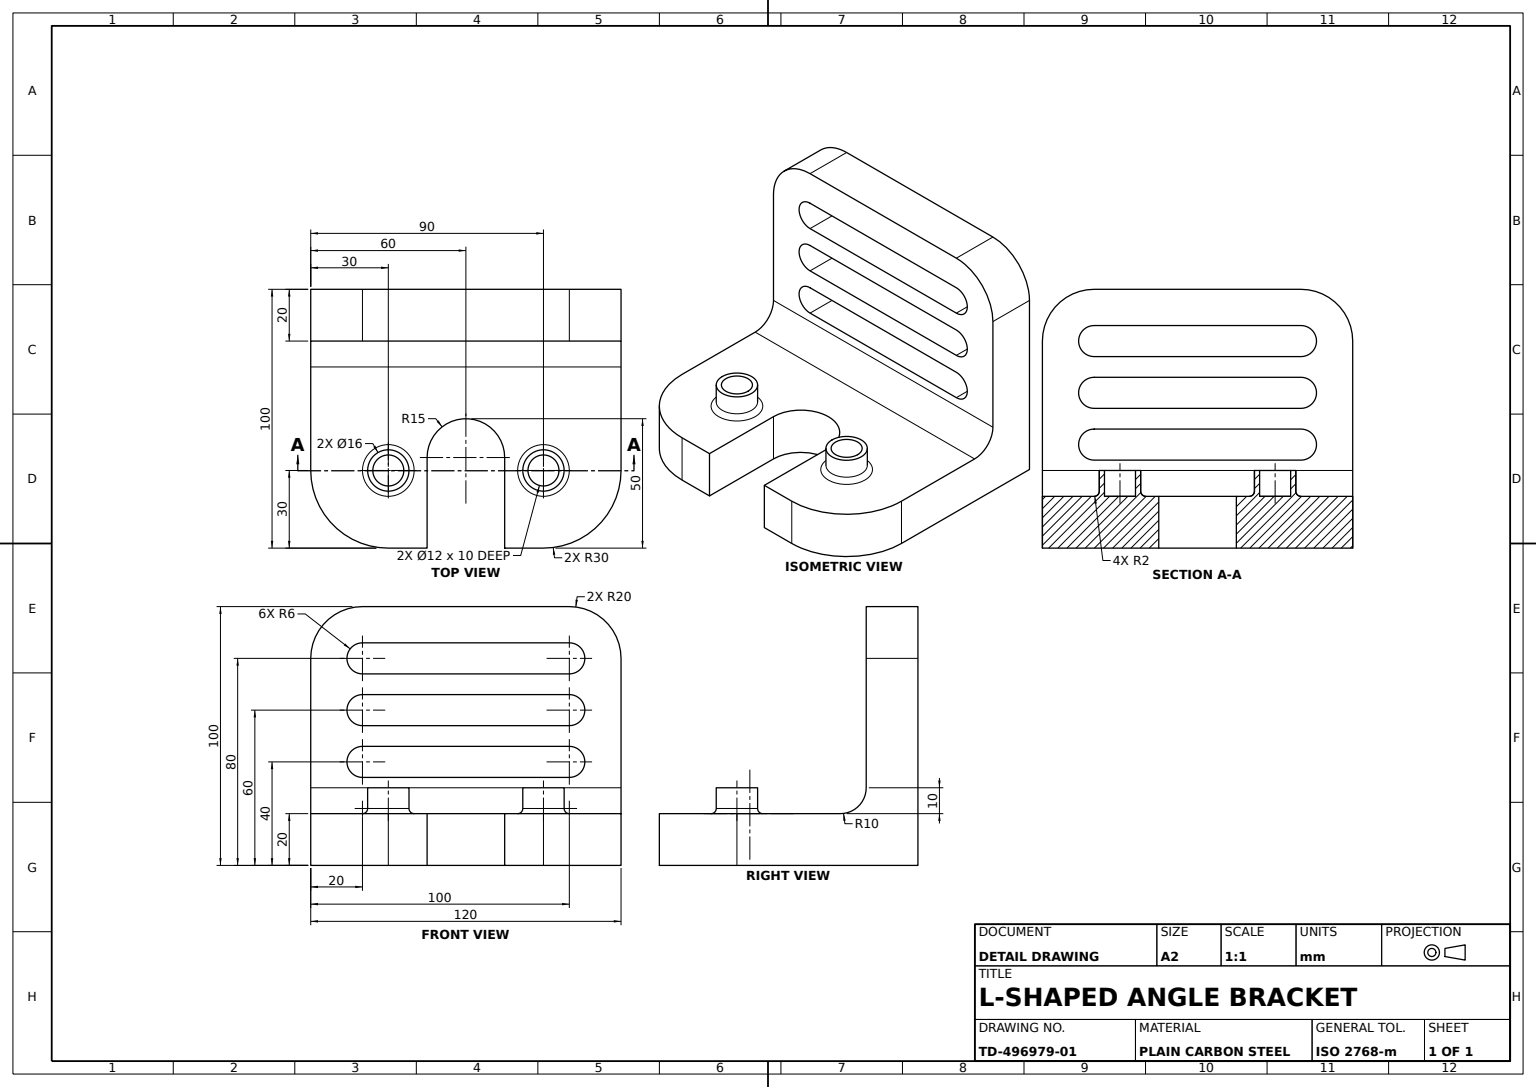
SolidWorks part; units mm, degrees
material "Plain Carbon Steel"
ref_plane "Front Plane" through (0, 0, 0) normal (0, 0, 1) x (1, 0, 0)
ref_plane "Top Plane" through (0, 0, 0) normal (0, 1, 0) x (1, 0, 0)
ref_plane "Right Plane" through (0, 0, 0) normal (1, 0, 0) x (0, 0, -1)
sketch "Bracket L Profile" plane through (0, 0, 0) normal (0, 0, 1) x (1, 0, 0)
  line L1 (0, 0) -> (20, 0)
  line L2 (0, 0) -> (0, -100)
  line L3 (0, -100) -> (20, -100)
  line L4 (20, 0) -> (20, -70)
  line L5 (0, -100) -> (100, -100)
  line L6 (0, -100) -> (0, -80)
  line L7 (30, -80) -> (100, -80)
  line L8 (100, -100) -> (100, -80)
  arc A0 (30, -80) -> (20, -70) centre (30, -70) cw
  dimension "D5" = 10
  dimension "D1" = 100
  dimension "D2" = 100
  dimension "D3" = 20
  dimension "D4" = 20
extrude "Bracket Body" add sketch "Bracket L Profile" along normal mid plane 120 contours L7 A0 L4 L1 L2 L3 L5 L8
fillet "Corner Fillet R30" radius 30 2 edges at (100, -90, -60) (100, -90, 60)
fillet "Corner Fillet R20" radius 20 2 edges at (10, 0, -60) (10, 0, 60)
sketch "Upright Slots Profile" plane through (20, 0, 0) normal (1, 0, 0) x (0, 0, -1)
  line L0 (-40, -20) -> (40, -20) construction
  line L1 (-40, -14) -> (40, -14)
  line L2 (-40, -26) -> (40, -26)
  line L3 (-40, 0) -> (40, 0) construction
  line L4 (-60, -20) -> (-60, -70) construction
  line L5 (-40, -46) -> (40, -46)
  line L6 (-40, -34) -> (40, -34)
  line L7 (-40, -40) -> (40, -40) construction
  line L8 (-40, -66) -> (40, -66)
  line L9 (-40, -54) -> (40, -54)
  line L10 (-40, -60) -> (40, -60) construction
  arc A0 (-40, -14) -> (-40, -26) centre (-40, -20) ccw
  arc A1 (40, -26) -> (40, -14) centre (40, -20) ccw
  arc A2 (-40, -34) -> (-40, -46) centre (-40, -40) ccw
  arc A3 (40, -46) -> (40, -34) centre (40, -40) ccw
  arc A4 (-40, -54) -> (-40, -66) centre (-40, -60) ccw
  arc A5 (40, -66) -> (40, -54) centre (40, -60) ccw
  point P2 (0, -20)
  point P16 (0, -40)
  point P23 (0, -60)
  dimension "D3" = 6
  dimension "D1" = 20
  dimension "D2" = 20
  dimension "D5" = 20
  dimension "D4" = 3
sketch "Base Notch Profile" plane through (0, -80, 0) normal (0, 1, 0) x (1, 0, 0)
  line L0 (65, 15) -> (100, 15)
  line L1 (100, -30) -> (100, 30) construction
  line L2 (100, 15) -> (100, -15)
  line L3 (100, -15) -> (65, -15)
  arc A1 (65, -15) -> (65, 15) centre (65, 0) cw
  point P4 (100, 0)
  dimension "D4" = 15
  dimension "D1" = 35
  dimension "D2" = 30
  dimension "D3" = 35
extrude "Base Notch" cut sketch "Base Notch Profile" against normal blind 78
extrude "Upright Slots 3x" cut sketch "Upright Slots Profile" against normal blind 20
sketch "Base Bosses Profile" plane through (0, -80, 0) normal (0, 1, 0) x (1, 0, 0)
  line L0 (30, 60) -> (70, 60) construction
  line L1 (30, -60) -> (70, -60) construction
  line L2 (100, 15) -> (100, 30) construction
  circle A0 centre (70, 30) radius 8
  circle A1 centre (70, -30) radius 8
  dimension "D4" = 16
  dimension "D1" = 30
  dimension "D2" = 30
  dimension "D3" = 30
extrude "Base Bosses 2x" add sketch "Base Bosses Profile" along normal blind 10
fillet "Boss Edge Fillet R2" radius 2 2 edges at (70, -80, -22) (70, -80, 38)
sketch "Boss Holes Profile" plane through (0, -70, 0) normal (0, 1, 0) x (1, 0, 0)
  circle A0 centre (70, -30) radius 6
  circle A1 centre (70, 30) radius 6
  dimension "D1" = 12
  dimension "D2" = 12
extrude "Boss Holes 2x" cut sketch "Boss Holes Profile" against normal blind 10
